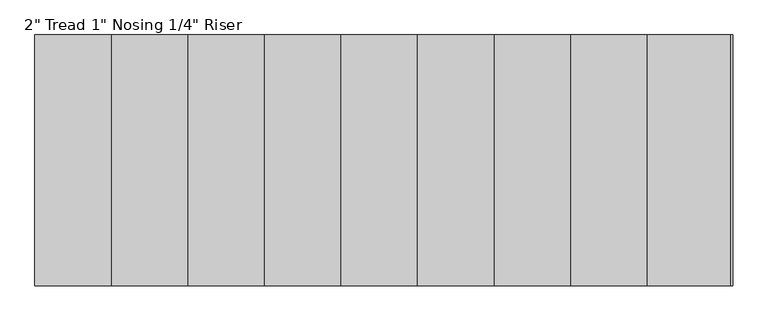
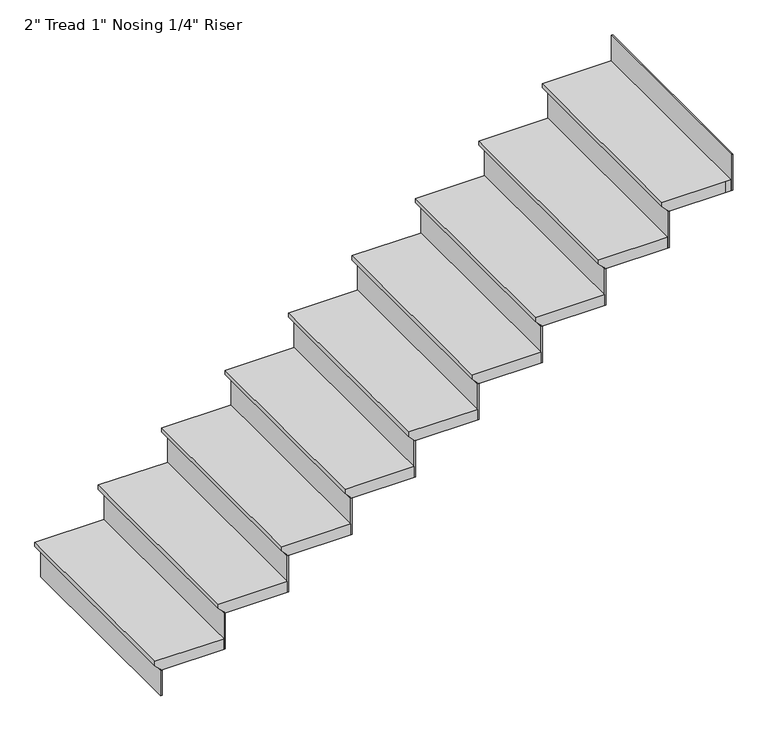
"""IFC4 building model written with IfcOpenShell, lengths in millimetres: stair flight geometry."""

from ifc_helpers import new_model, si_unit, origin, place, context, project, spatial, faceted_brep, source, transform, mapped, element, save


def stair_flight_b85e79d8(model_context):
    return source(origin(), model_context, "Body", "Brep", [
        faceted_brep([(-6516.8725091, 10512.3149226, 150.2833333), (-6516.8725091, 10512.3149226, 169.3333333), (-6516.8725091, 11426.7149226, 169.3333333), (-6516.8725091, 11426.7149226, 150.2833333), (-6491.4725091, 10512.3149226, 124.8833333), (-6491.4725091, 11426.7149226, 124.8833333), (-6212.0725091, 10512.3149226, 169.3333333), (-6212.0725091, 11426.7149226, 169.3333333), (-6491.4725091, 11426.7149226, 118.5333333), (-6212.0725091, 11426.7149226, 118.5333333), (-6212.0725091, 10512.3149226, 118.5333333), (-6491.4725091, 10512.3149226, 118.5333333)], [[[0, 1, 2, 3]], [[4, 0, 3, 5]], [[2, 1, 6, 7]], [[8, 9, 10, 11]], [[2, 7, 9, 8, 5, 3]], [[8, 11, 4, 5]], [[6, 1, 0, 4, 11, 10]], [[7, 6, 10, 9]]]),
        faceted_brep([(-6491.4725091, 10512.3149226, 118.5333333), (-6491.4725091, 10512.3149226, 0.0), (-6485.1225091, 10512.3149226, 0.0), (-6485.1225091, 10512.3149226, 118.5333333), (-6491.4725091, 11426.7149226, 118.5333333), (-6485.1225091, 11426.7149226, 118.5333333), (-6485.1225091, 11426.7149226, 0.0), (-6491.4725091, 11426.7149226, 0.0)], [[[0, 1, 2, 3]], [[4, 5, 6, 7]], [[1, 0, 4, 7]], [[2, 1, 7, 6]], [[3, 2, 6, 5]], [[0, 3, 5, 4]]]),
        faceted_brep([(-6212.0725091, 10512.3149226, 287.8666667), (-6212.0725091, 10512.3149226, 118.5333333), (-6205.7225091, 10512.3149226, 118.5333333), (-6205.7225091, 10512.3149226, 287.8666667), (-6212.0725091, 11426.7149226, 287.8666667), (-6205.7225091, 11426.7149226, 287.8666667), (-6205.7225091, 11426.7149226, 118.5333333), (-6212.0725091, 11426.7149226, 118.5333333)], [[[0, 1, 2, 3]], [[4, 5, 6, 7]], [[1, 0, 4, 7]], [[2, 1, 7, 6]], [[3, 2, 6, 5]], [[0, 3, 5, 4]]]),
        faceted_brep([(-6237.4725091, 11426.7149226, 338.6666667), (-6237.4725091, 10512.3149226, 338.6666667), (-5932.6725091, 10512.3149226, 338.6666667), (-5932.6725091, 11426.7149226, 338.6666667), (-6212.0725091, 11426.7149226, 287.8666667), (-5932.6725091, 11426.7149226, 287.8666667), (-5932.6725091, 10512.3149226, 287.8666667), (-6212.0725091, 10512.3149226, 287.8666667), (-6212.0725091, 11426.7149226, 294.2166667), (-6237.4725091, 11426.7149226, 319.6166667), (-6212.0725091, 10512.3149226, 294.2166667), (-6237.4725091, 10512.3149226, 319.6166667)], [[[0, 1, 2, 3]], [[4, 5, 6, 7]], [[0, 3, 5, 4, 8, 9]], [[4, 7, 10, 8]], [[2, 1, 11, 10, 7, 6]], [[3, 2, 6, 5]], [[11, 1, 0, 9]], [[10, 11, 9, 8]]]),
        faceted_brep([(-5932.6725091, 10512.3149226, 457.2), (-5932.6725091, 10512.3149226, 287.8666667), (-5926.3225091, 10512.3149226, 287.8666667), (-5926.3225091, 10512.3149226, 457.2), (-5932.6725091, 11426.7149226, 457.2), (-5926.3225091, 11426.7149226, 457.2), (-5926.3225091, 11426.7149226, 287.8666667), (-5932.6725091, 11426.7149226, 287.8666667)], [[[0, 1, 2, 3]], [[4, 5, 6, 7]], [[1, 0, 4, 7]], [[2, 1, 7, 6]], [[3, 2, 6, 5]], [[0, 3, 5, 4]]]),
        faceted_brep([(-5958.0725091, 11426.7149226, 508.0), (-5958.0725091, 10512.3149226, 508.0), (-5653.2725091, 10512.3149226, 508.0), (-5653.2725091, 11426.7149226, 508.0), (-5932.6725091, 11426.7149226, 457.2), (-5653.2725091, 11426.7149226, 457.2), (-5653.2725091, 10512.3149226, 457.2), (-5932.6725091, 10512.3149226, 457.2), (-5932.6725091, 11426.7149226, 463.55), (-5958.0725091, 11426.7149226, 488.95), (-5932.6725091, 10512.3149226, 463.55), (-5958.0725091, 10512.3149226, 488.95)], [[[0, 1, 2, 3]], [[4, 5, 6, 7]], [[0, 3, 5, 4, 8, 9]], [[4, 7, 10, 8]], [[2, 1, 11, 10, 7, 6]], [[3, 2, 6, 5]], [[11, 1, 0, 9]], [[10, 11, 9, 8]]]),
        faceted_brep([(-5653.2725091, 10512.3149226, 626.5333333), (-5653.2725091, 10512.3149226, 457.2), (-5646.9225091, 10512.3149226, 457.2), (-5646.9225091, 10512.3149226, 626.5333333), (-5653.2725091, 11426.7149226, 626.5333333), (-5646.9225091, 11426.7149226, 626.5333333), (-5646.9225091, 11426.7149226, 457.2), (-5653.2725091, 11426.7149226, 457.2)], [[[0, 1, 2, 3]], [[4, 5, 6, 7]], [[1, 0, 4, 7]], [[2, 1, 7, 6]], [[3, 2, 6, 5]], [[0, 3, 5, 4]]]),
        faceted_brep([(-5678.6725091, 11426.7149226, 677.3333333), (-5678.6725091, 10512.3149226, 677.3333333), (-5373.8725091, 10512.3149226, 677.3333333), (-5373.8725091, 11426.7149226, 677.3333333), (-5653.2725091, 11426.7149226, 626.5333333), (-5373.8725091, 11426.7149226, 626.5333333), (-5373.8725091, 10512.3149226, 626.5333333), (-5653.2725091, 10512.3149226, 626.5333333), (-5653.2725091, 11426.7149226, 632.8833333), (-5678.6725091, 11426.7149226, 658.2833333), (-5653.2725091, 10512.3149226, 632.8833333), (-5678.6725091, 10512.3149226, 658.2833333)], [[[0, 1, 2, 3]], [[4, 5, 6, 7]], [[0, 3, 5, 4, 8, 9]], [[4, 7, 10, 8]], [[2, 1, 11, 10, 7, 6]], [[3, 2, 6, 5]], [[11, 1, 0, 9]], [[10, 11, 9, 8]]]),
        faceted_brep([(-5373.8725091, 10512.3149226, 795.8666667), (-5373.8725091, 10512.3149226, 626.5333333), (-5367.5225091, 10512.3149226, 626.5333333), (-5367.5225091, 10512.3149226, 795.8666667), (-5373.8725091, 11426.7149226, 795.8666667), (-5367.5225091, 11426.7149226, 795.8666667), (-5367.5225091, 11426.7149226, 626.5333333), (-5373.8725091, 11426.7149226, 626.5333333)], [[[0, 1, 2, 3]], [[4, 5, 6, 7]], [[1, 0, 4, 7]], [[2, 1, 7, 6]], [[3, 2, 6, 5]], [[0, 3, 5, 4]]]),
        faceted_brep([(-5399.2725091, 11426.7149226, 846.6666667), (-5399.2725091, 10512.3149226, 846.6666667), (-5094.4725091, 10512.3149226, 846.6666667), (-5094.4725091, 11426.7149226, 846.6666667), (-5373.8725091, 11426.7149226, 795.8666667), (-5094.4725091, 11426.7149226, 795.8666667), (-5094.4725091, 10512.3149226, 795.8666667), (-5373.8725091, 10512.3149226, 795.8666667), (-5373.8725091, 11426.7149226, 802.2166667), (-5399.2725091, 11426.7149226, 827.6166667), (-5373.8725091, 10512.3149226, 802.2166667), (-5399.2725091, 10512.3149226, 827.6166667)], [[[0, 1, 2, 3]], [[4, 5, 6, 7]], [[0, 3, 5, 4, 8, 9]], [[4, 7, 10, 8]], [[2, 1, 11, 10, 7, 6]], [[3, 2, 6, 5]], [[11, 1, 0, 9]], [[10, 11, 9, 8]]]),
        faceted_brep([(-5094.4725091, 10512.3149226, 965.2), (-5094.4725091, 10512.3149226, 795.8666667), (-5088.1225091, 10512.3149226, 795.8666667), (-5088.1225091, 10512.3149226, 965.2), (-5094.4725091, 11426.7149226, 965.2), (-5088.1225091, 11426.7149226, 965.2), (-5088.1225091, 11426.7149226, 795.8666667), (-5094.4725091, 11426.7149226, 795.8666667)], [[[0, 1, 2, 3]], [[4, 5, 6, 7]], [[1, 0, 4, 7]], [[2, 1, 7, 6]], [[3, 2, 6, 5]], [[0, 3, 5, 4]]]),
        faceted_brep([(-5119.8725091, 11426.7149226, 1016.0), (-5119.8725091, 10512.3149226, 1016.0), (-4815.0725091, 10512.3149226, 1016.0), (-4815.0725091, 11426.7149226, 1016.0), (-5094.4725091, 11426.7149226, 965.2), (-4815.0725091, 11426.7149226, 965.2), (-4815.0725091, 10512.3149226, 965.2), (-5094.4725091, 10512.3149226, 965.2), (-5094.4725091, 11426.7149226, 971.55), (-5119.8725091, 11426.7149226, 996.95), (-5094.4725091, 10512.3149226, 971.55), (-5119.8725091, 10512.3149226, 996.95)], [[[0, 1, 2, 3]], [[4, 5, 6, 7]], [[0, 3, 5, 4, 8, 9]], [[4, 7, 10, 8]], [[2, 1, 11, 10, 7, 6]], [[3, 2, 6, 5]], [[11, 1, 0, 9]], [[10, 11, 9, 8]]]),
        faceted_brep([(-4815.0725091, 10512.3149226, 1134.5333333), (-4815.0725091, 10512.3149226, 965.2), (-4808.7225091, 10512.3149226, 965.2), (-4808.7225091, 10512.3149226, 1134.5333333), (-4815.0725091, 11426.7149226, 1134.5333333), (-4808.7225091, 11426.7149226, 1134.5333333), (-4808.7225091, 11426.7149226, 965.2), (-4815.0725091, 11426.7149226, 965.2)], [[[0, 1, 2, 3]], [[4, 5, 6, 7]], [[1, 0, 4, 7]], [[2, 1, 7, 6]], [[3, 2, 6, 5]], [[0, 3, 5, 4]]]),
        faceted_brep([(-4840.4725091, 11426.7149226, 1185.3333333), (-4840.4725091, 10512.3149226, 1185.3333333), (-4535.6725091, 10512.3149226, 1185.3333333), (-4535.6725091, 11426.7149226, 1185.3333333), (-4815.0725091, 11426.7149226, 1134.5333333), (-4535.6725091, 11426.7149226, 1134.5333333), (-4535.6725091, 10512.3149226, 1134.5333333), (-4815.0725091, 10512.3149226, 1134.5333333), (-4815.0725091, 11426.7149226, 1140.8833333), (-4840.4725091, 11426.7149226, 1166.2833333), (-4815.0725091, 10512.3149226, 1140.8833333), (-4840.4725091, 10512.3149226, 1166.2833333)], [[[0, 1, 2, 3]], [[4, 5, 6, 7]], [[0, 3, 5, 4, 8, 9]], [[4, 7, 10, 8]], [[2, 1, 11, 10, 7, 6]], [[3, 2, 6, 5]], [[11, 1, 0, 9]], [[10, 11, 9, 8]]]),
        faceted_brep([(-4535.6725091, 10512.3149226, 1303.8666667), (-4535.6725091, 10512.3149226, 1134.5333333), (-4529.3225091, 10512.3149226, 1134.5333333), (-4529.3225091, 10512.3149226, 1303.8666667), (-4535.6725091, 11426.7149226, 1303.8666667), (-4529.3225091, 11426.7149226, 1303.8666667), (-4529.3225091, 11426.7149226, 1134.5333333), (-4535.6725091, 11426.7149226, 1134.5333333)], [[[0, 1, 2, 3]], [[4, 5, 6, 7]], [[1, 0, 4, 7]], [[2, 1, 7, 6]], [[3, 2, 6, 5]], [[0, 3, 5, 4]]]),
        faceted_brep([(-4561.0725091, 11426.7149226, 1354.6666667), (-4561.0725091, 10512.3149226, 1354.6666667), (-4256.2725091, 10512.3149226, 1354.6666667), (-4256.2725091, 11426.7149226, 1354.6666667), (-4535.6725091, 11426.7149226, 1303.8666667), (-4256.2725091, 11426.7149226, 1303.8666667), (-4256.2725091, 10512.3149226, 1303.8666667), (-4535.6725091, 10512.3149226, 1303.8666667), (-4535.6725091, 11426.7149226, 1310.2166667), (-4561.0725091, 11426.7149226, 1335.6166667), (-4535.6725091, 10512.3149226, 1310.2166667), (-4561.0725091, 10512.3149226, 1335.6166667)], [[[0, 1, 2, 3]], [[4, 5, 6, 7]], [[0, 3, 5, 4, 8, 9]], [[4, 7, 10, 8]], [[2, 1, 11, 10, 7, 6]], [[3, 2, 6, 5]], [[11, 1, 0, 9]], [[10, 11, 9, 8]]]),
        faceted_brep([(-4256.2725091, 10512.3149226, 1473.2), (-4256.2725091, 10512.3149226, 1303.8666667), (-4249.9225091, 10512.3149226, 1303.8666667), (-4249.9225091, 10512.3149226, 1473.2), (-4256.2725091, 11426.7149226, 1473.2), (-4249.9225091, 11426.7149226, 1473.2), (-4249.9225091, 11426.7149226, 1303.8666667), (-4256.2725091, 11426.7149226, 1303.8666667)], [[[0, 1, 2, 3]], [[4, 5, 6, 7]], [[1, 0, 4, 7]], [[2, 1, 7, 6]], [[3, 2, 6, 5]], [[0, 3, 5, 4]]]),
        faceted_brep([(-3976.8725091, 10512.3149226, 1642.5333333), (-3976.8725091, 10512.3149226, 1473.2), (-3970.5225091, 10512.3149226, 1473.2), (-3970.5225091, 10512.3149226, 1642.5333333), (-3976.8725091, 11426.7149226, 1642.5333333), (-3970.5225091, 11426.7149226, 1642.5333333), (-3970.5225091, 11426.7149226, 1473.2), (-3976.8725091, 11426.7149226, 1473.2)], [[[0, 1, 2, 3]], [[4, 5, 6, 7]], [[1, 0, 4, 7]], [[2, 1, 7, 6]], [[3, 2, 6, 5]], [[0, 3, 5, 4]]]),
        faceted_brep([(-3976.8725091, 11426.7149226, 1524.0), (-4002.2725091, 11426.7149226, 1524.0), (-4281.6725091, 11426.7149226, 1524.0), (-4281.6725091, 10512.3149226, 1524.0), (-4002.2725091, 10512.3149226, 1524.0), (-3976.8725091, 10512.3149226, 1524.0), (-4002.2725091, 11426.7149226, 1473.2), (-3976.8725091, 11426.7149226, 1473.2), (-3976.8725091, 10512.3149226, 1473.2), (-4002.2725091, 10512.3149226, 1473.2), (-4256.2725091, 10512.3149226, 1473.2), (-4256.2725091, 11426.7149226, 1473.2), (-4256.2725091, 11426.7149226, 1479.55), (-4281.6725091, 11426.7149226, 1504.95), (-4256.2725091, 10512.3149226, 1479.55), (-4281.6725091, 10512.3149226, 1504.95)], [[[0, 1, 2, 3, 4, 5]], [[6, 7, 8, 9, 10, 11]], [[1, 0, 7, 6]], [[2, 1, 6, 11, 12, 13]], [[11, 10, 14, 12]], [[4, 3, 15, 14, 10, 9]], [[5, 4, 9, 8]], [[0, 5, 8, 7]], [[15, 3, 2, 13]], [[14, 15, 13, 12]]]),
    ])


if __name__ == "__main__":
    model = new_model("IFC4")
    model_context = context("Model", 3, world=origin())
    ifc_project = project(units=[si_unit("LENGTHUNIT", "METRE", prefix="MILLI")], contexts=[model_context])
    site = spatial("IfcSite", under=ifc_project)
    building = spatial("IfcBuilding", under=site)
    placement = place(None, origin())
    stair_flight_shape = stair_flight_b85e79d8(model_context)
    element("IfcStairFlight", 1, ObjectType="2\" Tread 1\" Nosing 1/4\" Riser", at=placement, inside=building, context=model_context, shape_type="MappedRepresentation", body=[
        mapped(stair_flight_shape, transform((0.0, 0.0, 0.0), x_axis=(1.0, 0.0, 0.0), y_axis=(0.0, 1.0, 0.0), z_axis=(0.0, 0.0, 1.0))),
    ])
    save(model, "model.ifc")
